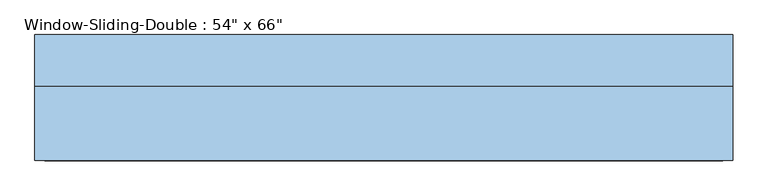
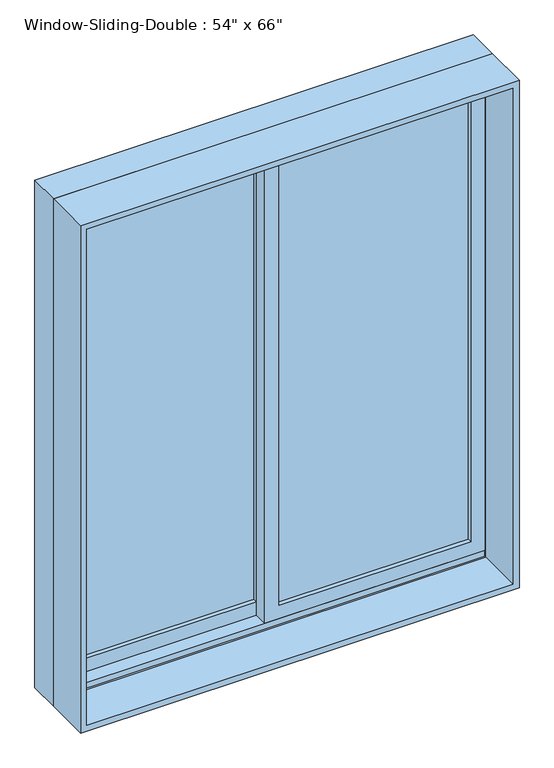
"""IFC4 building model written with IfcOpenShell, lengths in millimetres: window geometry."""

from ifc_helpers import new_model, si_unit, frame, origin, place, context, project, spatial, polyline, outline, extrude, faceted_brep, source, transform, mapped, element, save


def window_5810691a(model_context):
    return source(origin(), model_context, "Body", "SolidModel", [
        extrude(outline(polyline([(952.5, 666.75), (2571.75, 666.75), (2571.75, -22.225), (952.5, -22.225), (952.5, 666.75)]), holes=[polyline([(996.95, 22.225), (2527.3, 22.225), (2527.3, 622.3), (996.95, 622.3), (996.95, 22.225)])]), frame((0.0, 34.29, 0.0), z_axis=(0.0, 1.0, 0.0), x_axis=(0.0, 0.0, 1.0)), (0.0, 0.0, 1.0), 44.45),
        extrude(outline(polyline([(933.45, -666.75), (933.45, 22.225), (2571.75, 22.225), (2571.75, -666.75), (933.45, -666.75)]), holes=[polyline([(2527.3, -22.225), (996.95, -22.225), (996.95, -622.3), (2527.3, -622.3), (2527.3, -22.225)])]), frame((0.0, 78.74, 0.0), z_axis=(0.0, 1.0, 0.0), x_axis=(0.0, 0.0, 1.0)), (0.0, 0.0, 1.0), 44.45),
        extrude(outline(polyline([(-22.225, 110.49), (-22.225, 104.14), (-622.3, 104.14), (-622.3, 110.49), (-22.225, 110.49)])), frame((0.0, 0.0, 996.95), z_axis=(0.0, 0.0, 1.0), x_axis=(1.0, 0.0, 0.0)), (0.0, 0.0, 1.0), 1530.35),
        extrude(outline(polyline([(-22.225, 97.79), (-22.225, 91.44), (-622.3, 91.44), (-622.3, 97.79), (-22.225, 97.79)])), frame((0.0, 0.0, 996.95), z_axis=(0.0, 0.0, 1.0), x_axis=(1.0, 0.0, 0.0)), (0.0, 0.0, 1.0), 1530.35),
        extrude(outline(polyline([(622.3, 66.04), (622.3, 59.69), (22.225, 59.69), (22.225, 66.04), (622.3, 66.04)])), frame((0.0, 0.0, 996.95), z_axis=(0.0, 0.0, 1.0), x_axis=(1.0, 0.0, 0.0)), (0.0, 0.0, 1.0), 1530.35),
        extrude(outline(polyline([(622.3, 53.34), (622.3, 46.99), (22.225, 46.99), (22.225, 53.34), (622.3, 53.34)])), frame((0.0, 0.0, 996.95), z_axis=(0.0, 0.0, 1.0), x_axis=(1.0, 0.0, 0.0)), (0.0, 0.0, 1.0), 1530.35),
        extrude(outline(polyline([(2590.8, -685.8), (914.4, -685.8), (914.4, 685.8), (2590.8, 685.8), (2590.8, -685.8)]), holes=[polyline([(2571.75, 666.75), (933.45, 666.75), (933.45, -666.75), (2571.75, -666.75), (2571.75, 666.75)])]), frame((0.0, -118.11, 0.0), z_axis=(0.0, 1.0, 0.0), x_axis=(0.0, 0.0, 1.0)), (0.0, 0.0, 1.0), 146.05),
        faceted_brep([(-685.8, 27.94, 914.4), (-685.8, 129.54, 914.4), (685.8, 129.54, 914.4), (685.8, 27.94, 914.4), (-644.8778905, 129.54, 2549.8778905), (-644.8778905, 123.19, 2549.8778905), (-644.8778905, 123.19, 933.45), (-644.8778905, 129.54, 933.45), (644.8778905, 123.19, 2549.8778905), (644.8778905, 123.19, 933.45), (666.75, 123.19, 933.45), (666.75, 123.19, 2571.75), (-666.75, 123.19, 2571.75), (-666.75, 123.19, 933.45), (-666.75, 27.94, 2571.75), (-666.75, 27.94, 933.45), (-666.75, 34.29, 933.45), (-666.75, 34.29, 952.5), (-666.75, 78.74, 952.5), (-666.75, 78.74, 933.45), (685.8, 27.94, 2590.8), (-685.8, 27.94, 2590.8), (666.75, 27.94, 2571.75), (666.75, 27.94, 933.45), (-685.8, 129.54, 2590.8), (685.8, 129.54, 2590.8), (644.8778905, 129.54, 933.45), (644.8778905, 129.54, 2549.8778905), (666.75, 78.74, 933.45), (666.75, 78.74, 952.5), (666.75, 34.29, 952.5), (666.75, 34.29, 933.45)], [[[0, 1, 2, 3]], [[4, 5, 6, 7]], [[5, 8, 9, 10, 11, 12, 13, 6]], [[12, 14, 15, 16, 17, 18, 19, 13]], [[0, 3, 20, 21], [22, 23, 15, 14]], [[24, 1, 0, 21]], [[2, 1, 24, 25], [4, 7, 26, 27]], [[5, 4, 27, 8]], [[12, 11, 22, 14]], [[21, 20, 25, 24]], [[8, 27, 26, 9]], [[22, 11, 10, 28, 29, 30, 31, 23]], [[20, 3, 2, 25]], [[26, 7, 6, 13, 19, 28, 10, 9]], [[28, 19, 18, 29]], [[29, 18, 17, 30]], [[30, 17, 16, 31]], [[15, 23, 31, 16]]]),
    ])


if __name__ == "__main__":
    model = new_model("IFC4")
    model_context = context("Model", 3, world=origin())
    ifc_project = project(units=[si_unit("LENGTHUNIT", "METRE", prefix="MILLI")], contexts=[model_context])
    site = spatial("IfcSite", under=ifc_project)
    building = spatial("IfcBuilding", under=site)
    placement = place(None, origin())
    window_shape = window_5810691a(model_context)
    element("IfcWindow", 1, ObjectType="Window-Sliding-Double : 54\" x 66\"", at=placement, inside=building, context=model_context, shape_type="MappedRepresentation", body=[
        mapped(window_shape, transform((0.0, 0.0, 0.0), x_axis=(1.0, 0.0, 0.0), y_axis=(0.0, 1.0, 0.0), z_axis=(0.0, 0.0, 1.0))),
    ])
    save(model, "model.ifc")

# Revit data of these elements
# Type "Window-Sliding-Double : 54\" x 66\""
#   Type Mark = "20"
#   Fire Rating = "0.5h"
#   Assembly Code = "B2020100"
#   Analytic Construction = "Double glazing - domestic"
#   Window Inset [instance default] = 0' - 0"
#   Wall Thickness [instance default] = 0' - 6"
#   Visual Light Transmittance = 0.81
#   Thermal Resistance (R) = 1.8146 (h·ft²·°F)/BTU
#   Solar Heat Gain Coefficient = 0.76
#   Muntin Width = 1' - 11 5/8"
#   Muntin Height = 5' - 0 1/4"
#   Interior Wall Closure [instance default] = 0' - 2 3/4"
#   Heat Transfer Coefficient (U) = 0.5511 BTU/(h·ft²·°F)
#   Frame Extension [instance default] = 0' - 0 1/4"
#   Exterior Wall Closure [instance default] = 0' - 1 1/4"
#   Rough Width = 4' - 6 1/2"
#   Rough Height = 5' - 6 1/2"
#   Height = 5' - 6"
#   Extension Jamb [instance default] = 0' - 2 3/4"
#   Default Sill Height = 3' - 0"
#   Width = 4' - 6"
#   Interior Trim Visibility [instance default] = yes
#   Indicator Visibility [instance default] = yes
#   Exterior Trim Visibility [instance default] = yes
#   Muntin Visibility = yes
#   Extension Jamb Visibility [instance default] = yes
#   Muntin Pattern = Muntin Pattern_2x2 : Muntin Pattern_2x2
#   Interior Trim Material = Wood - Stained
#   Interior Trim = Trim-Window-Interior-Flat : Picture Frame
#   Interior Frame Material = Wood - Stained
#   Glass Panel Material = Glass
#   Exterior Trim Material = Clad - White
#   Exterior Trim = Trim-Window-Exterior-Flat : with Sill
#   Exterior Frame Material = Clad - White
#   Wall Closure = (empty or 0)
# Element 1 (IfcWindow, "Window-Sliding-Double : 54\" x 66\"")
#   Wall Thickness = 0' - 9"
#   Extension Jamb = 0' - 5 3/4"
#   Materials on its faces: "Wood - Stained", "Glass", "Clad - White"
# Materials
#   "Wood - Stained": class "Wood", colour RGB 224 178 126, transparency 0, Cost = 0
#   "Glass": class "Glass", colour RGB 0 128 192, transparency 0.75, Description = "Soda Lime Glass", Cost = 0
#   "Clad - White": class "Wood", colour RGB 242 242 238, transparency 0, Cost = 0
